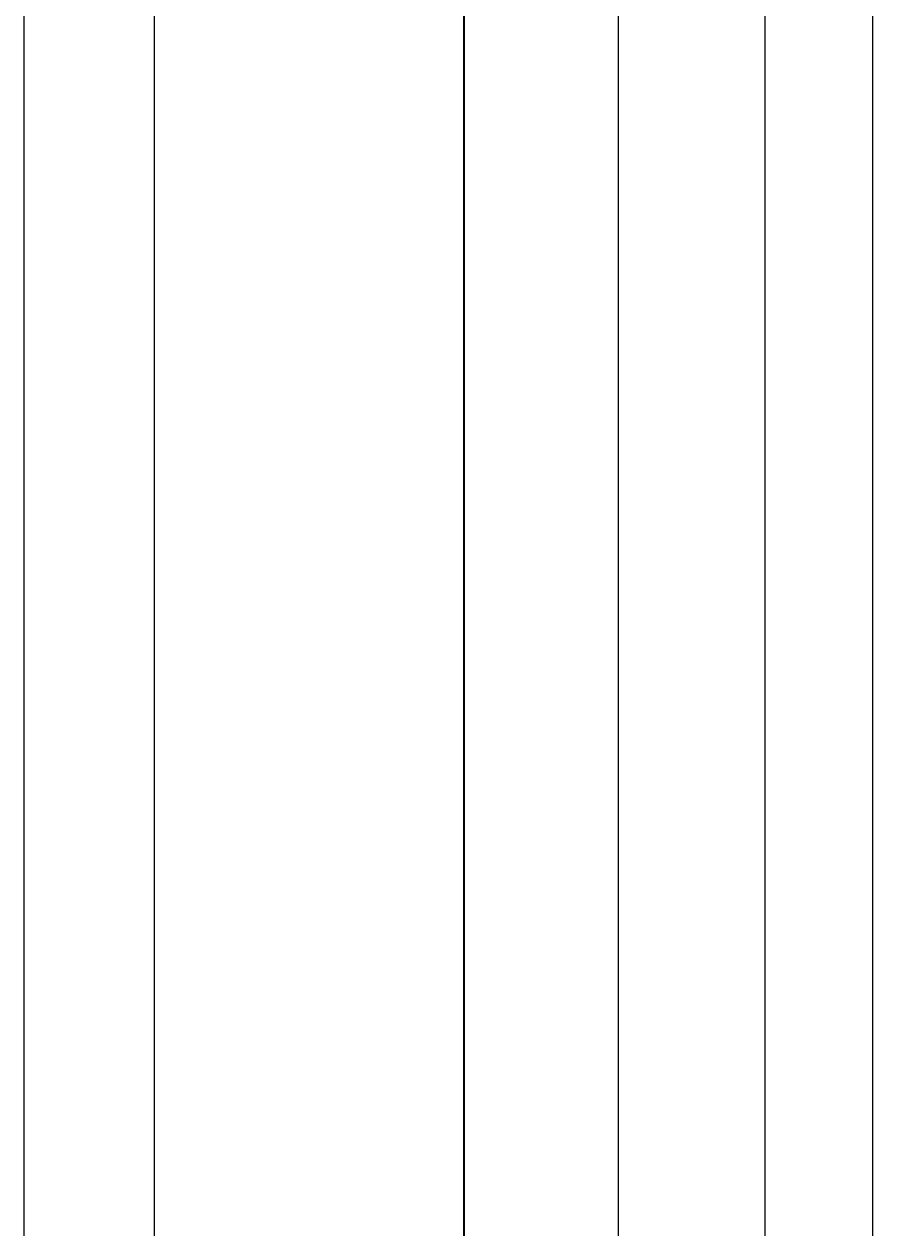
# Model space of a CAD drawing. Units: inches. Extents: x -6 to 289, y -8 to 323.
# Tile 58 of 107: x 107 to 124, y 206 to 229. Entities that reach past the tile are written whole.
import ezdxf

# ---------------------------------------------------------------- set-up
doc = ezdxf.new("R2010")
doc.units = ezdxf.units.IN
doc.header["$MEASUREMENT"] = 0
doc.layers.add('A-ANNO-DIMS', color=2, linetype='Continuous', lineweight=18)
doc.layers.add('A-ELEV', color=7, linetype='Continuous', lineweight=35)
doc.styles.get("Standard").update_dxf_attribs({"font": 'arial.ttf'})
doc.dimstyles.get("Standard").update_dxf_attribs({"dimtxt": 0.18, "dimasz": 0.18, "dimexe": 0.18, "dimexo": 0.0625, "dimgap": 0.09, "dimtad": 0, "dimtih": 1, "dimtoh": 1, "dimdec": 4, "dimzin": 0, "dimdsep": 46, "dimtxsty": 'Standard', "dimcen": 0.09, "dimadec": 0, "dimazin": 0, "dimtfac": 1, "dimtdec": 4, "dimtofl": 0, "dimtmove": 0, "dimatfit": 3, "dimfxl": 1, "dimtolj": 1, "dimtzin": 0, "dimarcsym": 0})

# ---------------------------------------------------------------- blocks, each defined once
blk = doc.blocks.new('*D10')
at = {"layer": 'A-ANNO-DIMS', "color": 0, "lineweight": -2, "transparency": 16777216}
for p, q in [((115.164, 307.351), (115.164, 322.969)), ((115.344, 322.789), (120.639, 322.789)), ((126.703, 322.789), (121.408, 322.789)), ((126.883, 226.717), (126.883, 322.969))]:
    blk.add_line(p, q, dxfattribs=at)
at = {"layer": 'A-ANNO-DIMS', "color": 0, "transparency": 16777216}
for points in [[(115.344, 322.819), (115.344, 322.759), (115.164, 322.789)], [(126.703, 322.819), (126.703, 322.759), (126.883, 322.789)]]:
    blk.add_solid(points, dxfattribs=at)
at = {"layer": 'Defpoints', "color": 0, "transparency": 16777216}
for p in [(126.883, 322.789), (115.164, 307.289), (126.883, 226.654)]:
    blk.add_point(p, dxfattribs=at)
at = {"layer": 'A-ANNO-DIMS', "color": 0, "transparency": 16777216, "insert": (121.024, 322.789), "char_height": 0.18, "attachment_point": 5}
blk.add_mtext('\\A1;11.72', dxfattribs=at)
blk = doc.blocks.new('*D58')
at = {"layer": 'A-ANNO-DIMS', "color": 0, "lineweight": -2, "transparency": 16777216}
for p, q in [((106.634, 68.495), (106.634, 322.969)), ((106.814, 322.789), (114.479, 322.789)), ((122.914, 322.789), (115.249, 322.789)), ((123.094, 68.495), (123.094, 322.969))]:
    blk.add_line(p, q, dxfattribs=at)
at = {"layer": 'A-ANNO-DIMS', "color": 0, "transparency": 16777216}
for points in [[(106.814, 322.819), (106.814, 322.759), (106.634, 322.789)], [(122.914, 322.819), (122.914, 322.759), (123.094, 322.789)]]:
    blk.add_solid(points, dxfattribs=at)
at = {"layer": 'Defpoints', "color": 0, "transparency": 16777216}
for p in [(123.094, 322.789), (106.634, 68.432), (123.094, 68.432)]:
    blk.add_point(p, dxfattribs=at)
at = {"layer": 'A-ANNO-DIMS', "color": 0, "transparency": 16777216, "insert": (114.864, 322.789), "char_height": 0.18, "attachment_point": 5}
blk.add_mtext('\\A1;16.46', dxfattribs=at)
blk = doc.blocks.new('*D73')
at = {"layer": 'A-ANNO-DIMS', "color": 0, "lineweight": -2, "transparency": 16777216}
for p, q in [((121.008, 51.148), (121.008, 322.969)), ((121.188, 322.789), (127.697, 322.789)), ((135.116, 322.789), (128.607, 322.789)), ((135.296, 51.148), (135.296, 322.969))]:
    blk.add_line(p, q, dxfattribs=at)
at = {"layer": 'A-ANNO-DIMS', "color": 0, "transparency": 16777216}
for points in [[(121.188, 322.819), (121.188, 322.759), (121.008, 322.789)], [(135.116, 322.819), (135.116, 322.759), (135.296, 322.789)]]:
    blk.add_solid(points, dxfattribs=at)
at = {"layer": 'Defpoints', "color": 0, "transparency": 16777216}
for p in [(135.296, 322.789), (121.008, 51.085), (135.296, 51.085)]:
    blk.add_point(p, dxfattribs=at)
at = {"layer": 'A-ANNO-DIMS', "color": 0, "transparency": 16777216, "insert": (128.152, 322.789), "char_height": 0.18, "attachment_point": 5}
blk.add_mtext('\\A1;14.288', dxfattribs=at)
blk = doc.blocks.new('*D92')
at = {"layer": 'A-ANNO-DIMS', "color": 0, "lineweight": -2, "transparency": 16777216}
for p, q in [((109.164, 127.351), (109.164, 322.969)), ((109.344, 322.789), (112.014, 322.789)), ((114.984, 322.789), (112.313, 322.789)), ((115.164, 162.411), (115.164, 322.969))]:
    blk.add_line(p, q, dxfattribs=at)
at = {"layer": 'A-ANNO-DIMS', "color": 0, "transparency": 16777216}
for points in [[(109.344, 322.819), (109.344, 322.759), (109.164, 322.789)], [(114.984, 322.819), (114.984, 322.759), (115.164, 322.789)]]:
    blk.add_solid(points, dxfattribs=at)
at = {"layer": 'Defpoints', "color": 0, "transparency": 16777216}
for p in [(115.164, 322.789), (115.164, 162.348), (109.164, 127.289)]:
    blk.add_point(p, dxfattribs=at)
at = {"layer": 'A-ANNO-DIMS', "color": 0, "transparency": 16777216, "insert": (112.164, 322.789), "char_height": 0.18, "attachment_point": 5}
blk.add_mtext('\\A1;6', dxfattribs=at)
blk = doc.blocks.new('*D93')
at = {"layer": 'A-ANNO-DIMS', "color": 0, "lineweight": -2, "transparency": 16777216}
for p, q in [((115.164, 162.411), (115.164, 322.969)), ((115.344, 322.789), (116.515, 322.789)), ((117.984, 322.789), (116.813, 322.789)), ((118.164, 159.411), (118.164, 322.969))]:
    blk.add_line(p, q, dxfattribs=at)
at = {"layer": 'A-ANNO-DIMS', "color": 0, "transparency": 16777216}
for points in [[(115.344, 322.819), (115.344, 322.759), (115.164, 322.789)], [(117.984, 322.819), (117.984, 322.759), (118.164, 322.789)]]:
    blk.add_solid(points, dxfattribs=at)
at = {"layer": 'Defpoints', "color": 0, "transparency": 16777216}
for p in [(118.164, 322.789), (115.164, 162.348), (118.164, 159.348)]:
    blk.add_point(p, dxfattribs=at)
at = {"layer": 'A-ANNO-DIMS', "color": 0, "transparency": 16777216, "insert": (116.664, 322.789), "char_height": 0.18, "attachment_point": 5}
blk.add_mtext('\\A1;3', dxfattribs=at)
blk = doc.blocks.new('*D94')
at = {"layer": 'A-ANNO-DIMS', "color": 0, "lineweight": -2, "transparency": 16777216}
for p, q in [((118.164, 159.411), (118.164, 322.969)), ((118.344, 322.789), (139.46, 322.789)), ((161.372, 322.789), (140.256, 322.789)), ((161.552, 159.411), (161.552, 322.969))]:
    blk.add_line(p, q, dxfattribs=at)
at = {"layer": 'A-ANNO-DIMS', "color": 0, "transparency": 16777216}
for points in [[(118.344, 322.819), (118.344, 322.759), (118.164, 322.789)], [(161.372, 322.819), (161.372, 322.759), (161.552, 322.789)]]:
    blk.add_solid(points, dxfattribs=at)
at = {"layer": 'Defpoints', "color": 0, "transparency": 16777216}
for p in [(161.552, 322.789), (118.164, 159.348), (161.552, 159.348)]:
    blk.add_point(p, dxfattribs=at)
at = {"layer": 'A-ANNO-DIMS', "color": 0, "transparency": 16777216, "insert": (139.858, 322.789), "char_height": 0.18, "attachment_point": 5}
blk.add_mtext('\\A1;43.39', dxfattribs=at)

msp = doc.modelspace()

# ---------------------------------------------------------------- linework, layer by layer
at = {"layer": 'A-ELEV'}
msp.add_line((115.1638, 247.2888), (115.1638, 139.2888), dxfattribs=at)

# ---------------------------------------------------------------- dimensions: what is measured, and where the dimension line sits
at = {"layer": 'A-ANNO-DIMS'}
for base, p1, p2, override, picture, middle in [((123.094, 322.7888), (106.634, 68.4322), (123.094, 68.4322), {"dimdec": 2, "dimlfac": 1, "dimrnd": 0, "dimzin": 0, "dimdsep": 46, "dimlunit": 2}, '*D58', (114.864, 322.7888)), ((115.1638, 322.7888), (109.1638, 127.2888), (115.1638, 162.3484), {"dimdec": 0, "dimlfac": 1, "dimrnd": 0, "dimzin": 0, "dimdsep": 46, "dimlunit": 2}, '*D92', (112.1638, 322.7888)), ((126.8835, 322.7888), (115.1638, 307.2888), (126.8835, 226.654), {"dimdec": 2, "dimlfac": 1, "dimrnd": 0, "dimzin": 0, "dimdsep": 46, "dimlunit": 2}, '*D10', (121.0236, 322.7888)), ((118.1638, 322.7888), (115.1638, 162.3484), (118.1638, 159.3484), {"dimdec": 0, "dimlfac": 1, "dimrnd": 0, "dimzin": 0, "dimdsep": 46, "dimlunit": 2}, '*D93', (116.6638, 322.7888)), ((161.5522, 322.7888), (118.1638, 159.3484), (161.5522, 159.3484), {"dimdec": 2, "dimlfac": 1, "dimrnd": 0, "dimzin": 0, "dimdsep": 46, "dimlunit": 2}, '*D94', (139.858, 322.7888)), ((135.296, 322.7888), (121.008, 51.0851), (135.296, 51.0851), {"dimdec": 3, "dimlfac": 1, "dimrnd": 0, "dimzin": 0, "dimdsep": 46, "dimlunit": 2}, '*D73', (128.152, 322.7888))]:
    dim = msp.add_linear_dim(base=base, p1=p1, p2=p2, dimstyle='Standard', override=override, dxfattribs=at)
    dim.commit()
    dim.dimension.update_dxf_attribs({"geometry": picture, "text_midpoint": middle})

doc.saveas('drawing.dxf')
